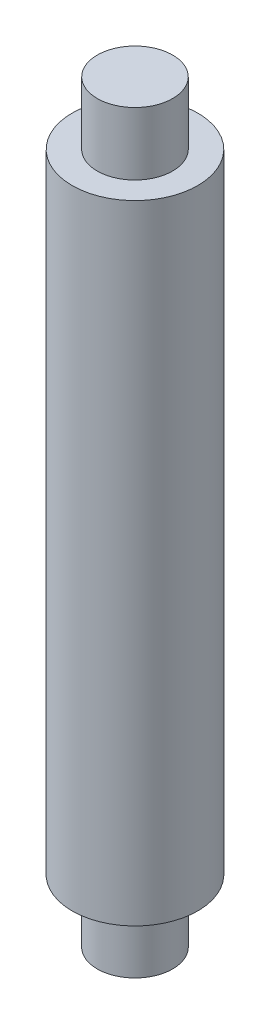
ISO-10303-21;
HEADER;
FILE_DESCRIPTION(('STEP AP214'),'2;1');
FILE_NAME('part.step','',(''),(''),'','','');
FILE_SCHEMA(('AUTOMOTIVE_DESIGN { 1 0 10303 214 1 1 1 1 }'));
ENDSEC;
DATA;
#1=APPLICATION_CONTEXT('core data for automotive mechanical design processes');
#2=APPLICATION_PROTOCOL_DEFINITION('international standard','automotive_design',2000,#1);
#3=PRODUCT_CONTEXT('',#1,'mechanical');
#4=PRODUCT('Part','Part','',(#3));
#5=PRODUCT_RELATED_PRODUCT_CATEGORY('part','',(#4));
#6=PRODUCT_DEFINITION_FORMATION('','',#4);
#7=PRODUCT_DEFINITION_CONTEXT('part definition',#1,'design');
#8=PRODUCT_DEFINITION('design','',#6,#7);
#9=PRODUCT_DEFINITION_SHAPE('','',#8);
#10=(LENGTH_UNIT() NAMED_UNIT(*) SI_UNIT(.MILLI.,.METRE.));
#11=(NAMED_UNIT(*) PLANE_ANGLE_UNIT() SI_UNIT($,.RADIAN.));
#12=(NAMED_UNIT(*) SI_UNIT($,.STERADIAN.) SOLID_ANGLE_UNIT());
#13=UNCERTAINTY_MEASURE_WITH_UNIT(LENGTH_MEASURE(1.E-05),#10,'distance_accuracy_value','');
#14=(GEOMETRIC_REPRESENTATION_CONTEXT(3) GLOBAL_UNCERTAINTY_ASSIGNED_CONTEXT((#13)) GLOBAL_UNIT_ASSIGNED_CONTEXT((#10,
#11,#12)) REPRESENTATION_CONTEXT('',''));
#15=CARTESIAN_POINT('',(0.,0.,0.));
#16=DIRECTION('',(0.,0.,1.));
#17=DIRECTION('',(1.,0.,0.));
#18=AXIS2_PLACEMENT_3D('',#15,#16,#17);
#19=CARTESIAN_POINT('',(0.,0.,0.));
#20=DIRECTION('',(0.,1.,0.));
#21=DIRECTION('',(0.,0.,1.));
#22=AXIS2_PLACEMENT_3D('',#19,#20,#21);
#23=PLANE('',#22);
#24=CARTESIAN_POINT('',(0.,0.,0.));
#25=DIRECTION('',(0.,1.,0.));
#26=DIRECTION('',(0.,0.,1.));
#27=AXIS2_PLACEMENT_3D('',#24,#25,#26);
#28=CIRCLE('',#27,6.);
#29=CARTESIAN_POINT('',(0.,0.,6.));
#30=VERTEX_POINT('',#29);
#31=EDGE_CURVE('E10',#30,#30,#28,.T.);
#32=ORIENTED_EDGE('',*,*,#31,.F.);
#33=EDGE_LOOP('',(#32));
#34=FACE_BOUND('',#33,.T.);
#35=ADVANCED_FACE('F40',(#34),#23,.F.);
#36=CARTESIAN_POINT('',(0.,120.,0.));
#37=DIRECTION('',(0.,1.,0.));
#38=DIRECTION('',(0.,0.,1.));
#39=AXIS2_PLACEMENT_3D('',#36,#37,#38);
#40=CYLINDRICAL_SURFACE('',#39,6.);
#41=CARTESIAN_POINT('',(0.,9.99999999999999,0.));
#42=DIRECTION('',(0.,1.,0.));
#43=DIRECTION('',(0.,0.,1.));
#44=AXIS2_PLACEMENT_3D('',#41,#42,#43);
#45=CIRCLE('',#44,6.);
#46=CARTESIAN_POINT('',(0.,9.99999999999999,6.));
#47=VERTEX_POINT('',#46);
#48=EDGE_CURVE('E43',#47,#47,#45,.T.);
#49=ORIENTED_EDGE('',*,*,#48,.F.);
#50=EDGE_LOOP('',(#49));
#51=FACE_BOUND('',#50,.T.);
#52=ORIENTED_EDGE('',*,*,#31,.T.);
#53=EDGE_LOOP('',(#52));
#54=FACE_BOUND('',#53,.T.);
#55=ADVANCED_FACE('F81',(#51,#54),#40,.T.);
#56=CARTESIAN_POINT('',(6.,10.,0.));
#57=DIRECTION('',(0.,1.,0.));
#58=DIRECTION('',(0.,0.,1.));
#59=AXIS2_PLACEMENT_3D('',#56,#57,#58);
#60=PLANE('',#59);
#61=CARTESIAN_POINT('',(0.,9.99999999999999,0.));
#62=DIRECTION('',(0.,1.,0.));
#63=DIRECTION('',(0.,0.,1.));
#64=AXIS2_PLACEMENT_3D('',#61,#62,#63);
#65=CIRCLE('',#64,10.);
#66=CARTESIAN_POINT('',(0.,9.99999999999999,10.));
#67=VERTEX_POINT('',#66);
#68=EDGE_CURVE('E50',#67,#67,#65,.T.);
#69=ORIENTED_EDGE('',*,*,#68,.F.);
#70=EDGE_LOOP('',(#69));
#71=FACE_BOUND('',#70,.T.);
#72=ORIENTED_EDGE('',*,*,#48,.T.);
#73=EDGE_LOOP('',(#72));
#74=FACE_BOUND('',#73,.T.);
#75=ADVANCED_FACE('F78',(#71,#74),#60,.F.);
#76=CARTESIAN_POINT('',(0.,120.,0.));
#77=DIRECTION('',(0.,1.,0.));
#78=DIRECTION('',(0.,0.,1.));
#79=AXIS2_PLACEMENT_3D('',#76,#77,#78);
#80=CYLINDRICAL_SURFACE('',#79,10.);
#81=CARTESIAN_POINT('',(0.,110.,0.));
#82=DIRECTION('',(0.,1.,0.));
#83=DIRECTION('',(0.,0.,1.));
#84=AXIS2_PLACEMENT_3D('',#81,#82,#83);
#85=CIRCLE('',#84,10.);
#86=CARTESIAN_POINT('',(0.,110.,10.));
#87=VERTEX_POINT('',#86);
#88=EDGE_CURVE('E51',#87,#87,#85,.T.);
#89=ORIENTED_EDGE('',*,*,#88,.F.);
#90=EDGE_LOOP('',(#89));
#91=FACE_BOUND('',#90,.T.);
#92=ORIENTED_EDGE('',*,*,#68,.T.);
#93=EDGE_LOOP('',(#92));
#94=FACE_BOUND('',#93,.T.);
#95=ADVANCED_FACE('F74',(#91,#94),#80,.T.);
#96=CARTESIAN_POINT('',(10.,110.,0.));
#97=DIRECTION('',(0.,-1.,0.));
#98=DIRECTION('',(0.,0.,-1.));
#99=AXIS2_PLACEMENT_3D('',#96,#97,#98);
#100=PLANE('',#99);
#101=CARTESIAN_POINT('',(0.,110.,0.));
#102=DIRECTION('',(0.,1.,0.));
#103=DIRECTION('',(0.,0.,1.));
#104=AXIS2_PLACEMENT_3D('',#101,#102,#103);
#105=CIRCLE('',#104,6.);
#106=CARTESIAN_POINT('',(0.,110.,6.));
#107=VERTEX_POINT('',#106);
#108=EDGE_CURVE('E57',#107,#107,#105,.T.);
#109=ORIENTED_EDGE('',*,*,#108,.F.);
#110=EDGE_LOOP('',(#109));
#111=FACE_BOUND('',#110,.T.);
#112=ORIENTED_EDGE('',*,*,#88,.T.);
#113=EDGE_LOOP('',(#112));
#114=FACE_BOUND('',#113,.T.);
#115=ADVANCED_FACE('F67',(#111,#114),#100,.F.);
#116=CARTESIAN_POINT('',(0.,120.,0.));
#117=DIRECTION('',(0.,1.,0.));
#118=DIRECTION('',(0.,0.,1.));
#119=AXIS2_PLACEMENT_3D('',#116,#117,#118);
#120=CYLINDRICAL_SURFACE('',#119,6.);
#121=CARTESIAN_POINT('',(0.,120.,0.));
#122=DIRECTION('',(0.,1.,0.));
#123=DIRECTION('',(0.,0.,1.));
#124=AXIS2_PLACEMENT_3D('',#121,#122,#123);
#125=CIRCLE('',#124,6.);
#126=CARTESIAN_POINT('',(0.,120.,6.));
#127=VERTEX_POINT('',#126);
#128=EDGE_CURVE('E56',#127,#127,#125,.T.);
#129=ORIENTED_EDGE('',*,*,#128,.F.);
#130=EDGE_LOOP('',(#129));
#131=FACE_BOUND('',#130,.T.);
#132=ORIENTED_EDGE('',*,*,#108,.T.);
#133=EDGE_LOOP('',(#132));
#134=FACE_BOUND('',#133,.T.);
#135=ADVANCED_FACE('F63',(#131,#134),#120,.T.);
#136=CARTESIAN_POINT('',(6.,120.,0.));
#137=DIRECTION('',(0.,-1.,0.));
#138=DIRECTION('',(0.,0.,-1.));
#139=AXIS2_PLACEMENT_3D('',#136,#137,#138);
#140=PLANE('',#139);
#141=ORIENTED_EDGE('',*,*,#128,.T.);
#142=EDGE_LOOP('',(#141));
#143=FACE_BOUND('',#142,.T.);
#144=ADVANCED_FACE('F64',(#143),#140,.F.);
#145=CLOSED_SHELL('',(#35,#55,#75,#95,#115,#135,#144));
#146=MANIFOLD_SOLID_BREP('B2',#145);
#147=ADVANCED_BREP_SHAPE_REPRESENTATION('',(#18,#146),#14);
#148=SHAPE_DEFINITION_REPRESENTATION(#9,#147);
ENDSEC;
END-ISO-10303-21;
